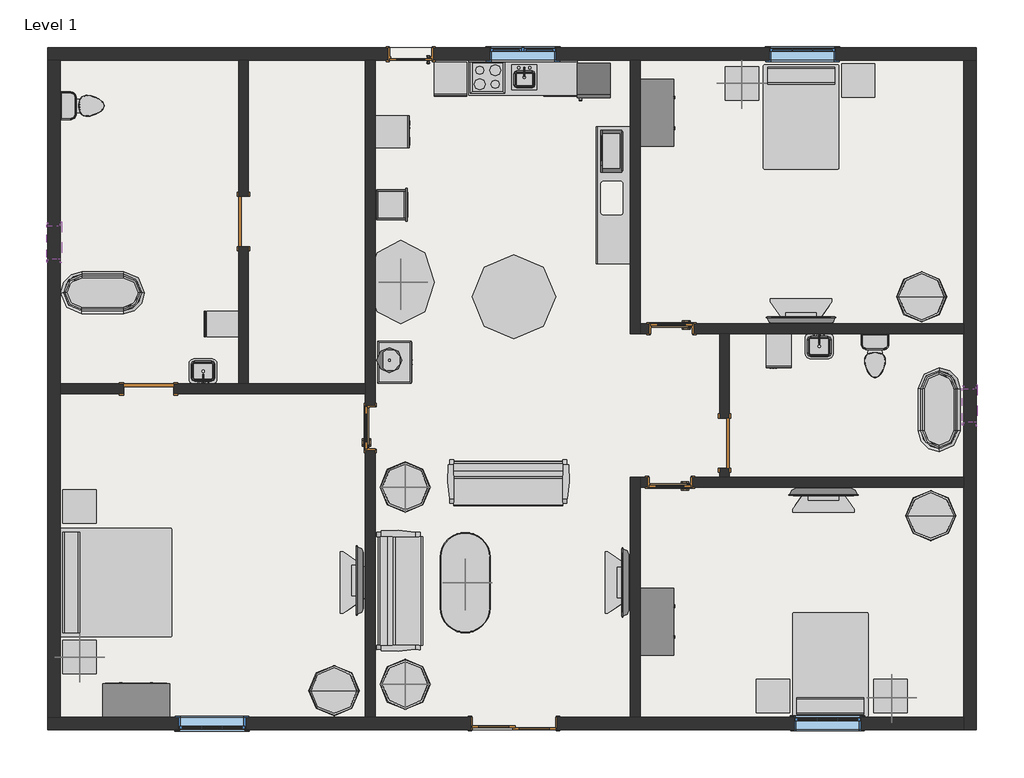
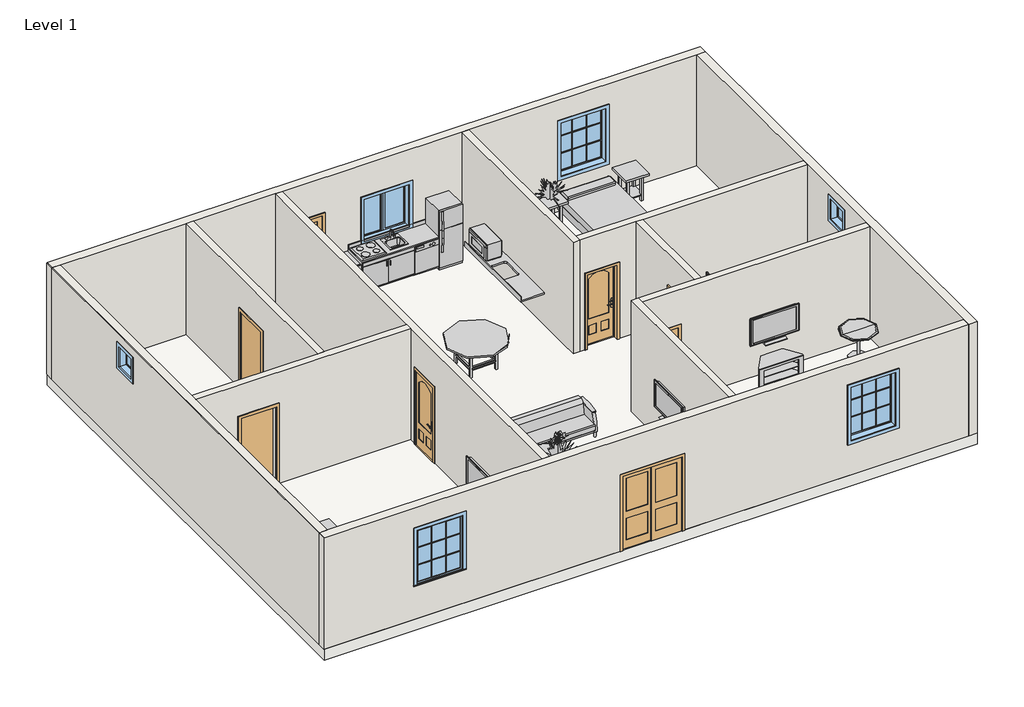
# One storey, incomplete: 33 furniture elements, 12 walls, 10 proxies, 8 doors, 8 flow terminals, 7 geographic elements, 6 windows, 1 slab.
# Revit data of these elements (continued)
# Type "Table-Dining Round w Chairs : 60\" Diameter" (continued)
#   Assembly Code = "E2020200"
#   Radius = 2' - 6"
#   Diameter = 5' - 0"
#   Height = 2' - 6"
#   Chairs = 6
#   Base Material = Pine
#   Top Material = Laminate, Linen, Matte
#   Default Elevation = 0
# Type "Table-Ellipse : 60\" x 48\""
#   Assembly Code = "E2020200"
#   Half Width = 2' - 0"
#   Half Length = 2' - 6"
#   Height = 2' - 6"
#   Length = 5' - 0"
#   Width = 4' - 0"
#   Base Material = Birch
#   Top Material = Birch
#   Default Elevation = 0
# Type "Table-Night Stand : 24\" x 24\" x 30\""
#   Assembly Code = "E2020200"
#   Depth = 2' - 0"
#   Height = 2' - 6"
#   Width = 2' - 0"
#   Base Material = Birch
#   Top Material = Laminate, Ivory, Matte
#   Default Elevation = 0
# Type "Table-Round : 36\" Diameter"
#   Assembly Code = "E2020200"
#   Base Radius = 0' - 10"
#   Height = 2' - 6"
#   Radius = 1' - 6"
#   Base Material = Steel, Chrome Plated
#   Top Material = Birch
#   Default Elevation = 0
# Type "RPC Plant - Tropical"
#   built-in parameter 1005198 = "{2, 15},{39, RPC-16-FWM5-GM7X-C67P-4000-ST1L-LVER-AU},{1, 0},{1, 0},{2, 13},{1, 8},{5, Color},{1, 0},{1, 0},{3, 0.8},{3, 0.8},{3, 0.8},{1, 8},{7, BBoxMin},{1, 0},{1, 0},{1, 0},{1, 0},{1, 0},{1, 8},{7, BBoxMax},{1, 0},{1, 0},{1, 0},{1, 0},{1, 0},{2, 11},{9, RPCTypeId},{1, 0},{1, 0},{39, RPC-16-FWM5-GM7X-C67P-4000-ST1L-LVER-AU},{1, 6},{14, RPCPlantHeight},{1, 0},{1, 0},{1, 3},{2, 11},{7, keyword},{1, 0},{1, 0},{35, :RPCs:Shrubs [General]:Geometry:RPC},{2, 11},{8, category},{1, 0},{1, 0},{16, Shrubs [General]},{2, 11},{12, LocalizedUID},{1, 0},{1, 0},{10, Crane Lily},{2, 14},{6, Height},{1, 0},{1, 0},{1, 3},{1, 2},{16, Cast Reflections},{1, 0},{1, 0},{1, 0},{1, 2},{12, Cast Shadows},{1, 0},{1, 0},{1, 1},{1, 2},{9, Lock View},{1, 0},{1, 0},{1, 0},{1, 4},{5, ViewC},{1, 0},{1, 0},{1, 0},{21, assetlibrary_base.fbx},{1, 5},"
#   built-in parameter 1005195 = "RPC-16-FWM5-GM7X-C67P-4000-ST1L-LVER-AU"
#   Assembly Code = "G2050500"
#   Height = 3' - 0"
#   Default Elevation = 0
# Type "RPC Plant - Tropical : Agave - 1.5'"
#   built-in parameter 1005198 = "{2, 15},{39, RPC-16-G1GJ-63FX-7K5P-N000-ST1L-LVER-AU},{1, 0},{1, 0},{2, 13},{1, 8},{5, Color},{1, 0},{1, 0},{3, 0.8},{3, 0.8},{3, 0.8},{1, 8},{7, BBoxMin},{1, 0},{1, 0},{1, 0},{1, 0},{1, 0},{1, 8},{7, BBoxMax},{1, 0},{1, 0},{1, 0},{1, 0},{1, 0},{2, 11},{9, RPCTypeId},{1, 0},{1, 0},{39, RPC-16-G1GJ-63FX-7K5P-N000-ST1L-LVER-AU},{1, 6},{14, RPCPlantHeight},{1, 0},{1, 0},{3, 1.5},{2, 11},{7, keyword},{1, 0},{1, 0},{35, :RPCs:Plants [General]:Geometry:RPC},{2, 11},{8, category},{1, 0},{1, 0},{16, Plants [General]},{2, 11},{12, LocalizedUID},{1, 0},{1, 0},{5, Agave},{2, 14},{6, Height},{1, 0},{1, 0},{3, 1.5},{1, 2},{16, Cast Reflections},{1, 0},{1, 0},{1, 0},{1, 2},{12, Cast Shadows},{1, 0},{1, 0},{1, 1},{1, 2},{9, Lock View},{1, 0},{1, 0},{1, 0},{1, 4},{5, ViewC},{1, 0},{1, 0},{1, 0},{21, assetlibrary_base.fbx},{1, 5},"
#   built-in parameter 1005195 = "RPC-16-G1GJ-63FX-7K5P-N000-ST1L-LVER-AU"
#   Type Comments = "Agave"
#   Assembly Code = "G2050500"
#   Height = 1' - 6"
#   Default Elevation = 0
# Type "Generic - 12\""
#   Assembly Code = "B1010"
#   Function = 0
#   Layers, outside or top first: 1' - 0" no material (function 1)
# Type "Generic - 8\""
#   Assembly Code = "B2010"
#   Layers, outside or top first: 0' - 9" "Brick, Common" (function 1)
# Type "INNER WALLS"
#   Assembly Code = "B2010"
#   Layers, outside or top first: 0' - 7" "Brick, Common" (function 1)
# Type "Casement 3x3 with Trim : 48\" x 60\""
#   Type Mark = "12"
#   Construction Type Id = "GSP4R"
#   Assembly Code = "B2020100"
#   Analytic Construction = "1/8 in Pilkington single glazing"
#   Visual Light Transmittance = 0.9
#   Solar Heat Gain Coefficient = 0.78
#   Heat Transfer Coefficient (U) = 0.6496 BTU/(h·ft²·°F)
#   Height = 5' - 0"
#   Default Sill Height = 1' - 0"
#   Trim Projection - Ext. = 0' - 0 1/2"
#   Trim Projection - Int. = 0' - 0 3/4"
#   Trim Width - Exterior = 0' - 3 1/2"
#   Trim Width - Interior = 0' - 3 1/2"
#   Width = 4' - 0"
#   Window Inset = 0' - 0 3/4"
#   Define Thermal Properties by = 1
#   Glass Pane Material = Glass
#   Sash Material = Sash
#   Trim Exterior Material = Trim
#   Trim Interior Material = Trim
#   Wall Closure = (empty or 0)
# Type "Casement Dbl with Trim : 48\" x 48\""
#   Type Mark = "13"
#   Construction Type Id = "GSP4R"
#   Assembly Code = "B2020100"
#   Analytic Construction = "1/8 in Pilkington single glazing"
#   Visual Light Transmittance = 0.9
#   Solar Heat Gain Coefficient = 0.78
#   Heat Transfer Coefficient (U) = 0.6496 BTU/(h·ft²·°F)
#   Height = 4' - 0"
#   Default Sill Height = 3' - 0"
#   Trim Projection - Ext. = 0' - 0 1/2"
#   Trim Projection - Int. = 0' - 0 3/4"
#   Trim Width - Exterior = 0' - 3 1/2"
#   Trim Width - Interior = 0' - 3 1/2"
#   Width = 4' - 0"
#   Window Inset = 0' - 0 3/4"
#   Define Thermal Properties by = 1
#   Glass Pane Material = Glass
#   Sash Material = Sash
#   Trim Exterior Material = Trim
#   Trim Interior Material = Trim
#   Wall Closure = (empty or 0)
# Type "Transom with Trim : 24\" x 24\""
#   Type Mark = "16"
#   Construction Type Id = "GSP4R"
#   Assembly Code = "B2020100"
#   Analytic Construction = "1/8 in Pilkington single glazing"
#   Visual Light Transmittance = 0.9
#   Solar Heat Gain Coefficient = 0.78
#   Heat Transfer Coefficient (U) = 0.6496 BTU/(h·ft²·°F)
#   Height = 2' - 0"
#   Default Sill Height = 7' - 1"
#   Trim Projection - Ext. = 0' - 0 1/2"
#   Trim Projection - Int. = 0' - 0 3/4"
#   Trim Width - Exterior = 0' - 3 1/2"
#   Trim Width - Interior = 0' - 3 1/2"
#   Width = 2' - 0"
#   Window Inset = 0' - 0 3/4"
#   Define Thermal Properties by = 1
#   Glass Pane Material = Glass
#   Sash Material = Sash
#   Trim Exterior Material = Trim
#   Trim Interior Material = Trim
#   Wall Closure = (empty or 0)
# Elements 1, 2 (IfcBuildingElementProxy, "18\" x 24\" x 34 1/2\"")
#   Phase Created = New Construction
#   Materials on its faces: "Steel, Paint Finish, Ivory, Matte", "Plastic, Opaque Black"
# Element 3 (IfcBuildingElementProxy, "Cook Top-4 Unit2 : 22\" x 20\"")
#   Phase Created = New Construction
#   Materials on its faces: "Steel, Chrome Plated", "Steel, Polished"
# Elements 4, 5 (IfcBuildingElementProxy, "Dishwasher : 23\" x 23 11/16\" x 33 1/2\"")
#   Phase Created = New Construction
#   Materials on its faces: "Steel, Paint Finish, Ivory, Glossy", "Plastic, Opaque Black"
# Element 6 (IfcBuildingElementProxy, "Dishwasher : 24\" x 24\" x 34\"")
#   Phase Created = New Construction
#   Materials on its faces: "Steel, Paint Finish, Ivory, Glossy", "Plastic, Opaque Black"
# Element 7 (IfcBuildingElementProxy, "Kitchenette - Medium : Kitchenette - Medium")
#   Phase Created = New Construction
#   Materials on its faces: "Cabinets", "Cabinets - Handles"
# Element 8 (IfcBuildingElementProxy, "Microwave : 30\" x 16\" x 18\"")
#   Phase Created = New Construction
#   Materials on its faces: "Laminate, Ivory, Matte", "Glass"
# Element 9 (IfcBuildingElementProxy, "Oven Double-Built-in : 21 1/2\" x 39 1/4\" x 21\"")
#   Phase Created = New Construction
#   Materials on its faces: "Steel", "Metal - Stainless Steel, Polished", "Glass"
# Element 10 (IfcBuildingElementProxy, "Refrigerator : 24\" x 25\" LH")
#   Phase Created = New Construction
#   Materials on its faces: "Steel, Paint Finish, Ivory, Glossy", "Steel, Chrome Plated"
# Elements 11, 12, 13 (IfcDoor, "30\" x 80\"")
#   Threshold Offset = 0' - 0 1/2"
#   Swing Angle = 90.00°
#   Door Offset = 0' - 0"
#   Threshold = yes
#   Exterior Trim = yes
#   Phase Created = New Construction
#   Materials on its faces: "Cherry", "Aluminum", "Glass"
# Element 14 (IfcDoor, "Door-Interior-Double-Sliding-2_Panel-Wood : 60\" x 80\"")
#   Phase Created = New Construction
#   Materials on its faces: "Cherry"
# Element 15 (IfcDoor, "Door-Interior-Single-Full Glass-Wood : 30\" x 80\"")
#   Swing Angle = 90.00°
#   Show Grill = yes
#   Phase Created = New Construction
#   Materials on its faces: "Cherry", "Aluminum", "Glass"
# Elements 16, 17, 18 (IfcDoor, "Single-Flush : 36\" x 84\"")
#   Phase Created = New Construction
#   Materials on its faces: "Door - Frame", "Door - Panel"
# Element 19 (IfcFlowTerminal, "Sink Kitchen-Island : 18\" x 18\"")
#   Mark = "10"
#   Phase Created = New Construction
#   Materials on its faces: "Steel, Polished"
# Element 20 (IfcFlowTerminal, "Sink Vanity-Round : 19\" x 19\"")
#   Mark = "11"
#   Phase Created = New Construction
#   Materials on its faces: "Porcelain, Linen", "Steel, Polished"
# Element 21 (IfcFlowTerminal, "Sink Vanity-Square : 20\" x 18\"")
#   Mark = "1"
#   Phase Created = New Construction
#   Materials on its faces: "Porcelain, Linen", "Steel, Polished"
# Element 22 (IfcFlowTerminal, "Sink Vanity-Square : 20\" x 18\"")
#   Mark = "9"
#   Phase Created = New Construction
#   Materials on its faces: "Porcelain, Linen", "Steel, Polished"
# Element 23 (IfcFlowTerminal, "Toilet-Domestic-3D : Toilet-Domestic-3D")
#   Mark = "2"
#   Phase Created = New Construction
#   Materials on its faces: "Porcelain, Linen", "Laminate, Linen, Matte"
# Element 24 (IfcFlowTerminal, "Toilet-Domestic-3D : Toilet-Domestic-3D")
#   Mark = "8"
#   Phase Created = New Construction
#   Materials on its faces: "Porcelain, Linen", "Laminate, Linen, Matte"
# Element 25 (IfcFlowTerminal, "Tub-Free Standing-3D : 30\" x 60\"")
#   Mark = "6"
#   Phase Created = New Construction
#   Materials on its faces: "Porcelain, Ivory"
# Element 26 (IfcFlowTerminal, "Tub-Free Standing-3D : 30\" x 60\"")
#   Mark = "7"
#   Phase Created = New Construction
#   Materials on its faces: "Porcelain, Ivory"
# Element 27 (IfcFurniture, "Base Cabinet-Double Door Sink Unit : 30\"")
#   Phase Created = New Construction
#   Materials on its faces: "Cabinets", "Cabinets - Handles"
# Elements 28, 29 (IfcFurniture, "Bed-Standard.0001 : Double 54\" x 75\"")
#   Phase Created = New Construction
#   Materials on its faces: "Linen, White", "Steel, Chrome Plated"
# Element 30 (IfcFurniture, "Bed-Standard.0001 : King 78\" x 80\"")
#   Phase Created = New Construction
#   Materials on its faces: "Linen, White", "Steel, Chrome Plated"
# Element 31 (IfcFurniture, "Counter Top w Sink Hole : 0600mm Depth")
#   Sink Opening Width = 1' - 11 1/8"
#   Sink Opening Depth = 1' - 2 7/8"
#   Sink Location To Wall = 0' - 3 15/16"
#   Sink Location = 3' - 11 1/4"
#   Length = 8' - 2 7/16"
#   Phase Created = New Construction
#   Materials on its faces: "Counter Top"
# Element 32 (IfcFurniture, "Counter Top w Sink Hole : 24\" Depth")
#   Sink Opening Depth = 1' - 2"
#   Sink Location To Wall = 0' - 6"
#   Length = 6' - 6"
#   Sink Location = 3' - 4"
#   Sink Opening Width = 1' - 4"
#   Phase Created = New Construction
#   Materials on its faces: "Counter Top"
# Elements 33, 34, 35 (IfcFurniture, "Dresser : 48\" x 72\" x 24\"")
#   Phase Created = New Construction
#   Materials on its faces: "Laminate, Ivory, Matte", "Cherry", "Laminate - Ivory, Glossy"
# Elements 36, 37 (IfcFurniture, "Sofa-Pensi : 84\"")
#   Phase Created = New Construction
#   Materials on its faces: "Cherry", "Linen, Beige", "Steel, Chrome Plated"
# Elements 38, 39, 40, 41 (IfcFurniture, "TV - Flat Screen : 50\"")
#   Stand = yes
#   Phase Created = New Construction
#   Materials on its faces: "TV - Black", "TV - Glass", "TV - Screen"
# Elements 42, 43, 44, 45 (IfcFurniture, "TV Stand : TV Stand")
#   Phase Created = New Construction
#   Materials on its faces: "Melamine - Gray", "Glass - Shelves"
# Element 46 (IfcFurniture, "Table-Dining Oval : 36\" x 72\"")
#   Phase Created = New Construction
#   Materials on its faces: "Steel, Chrome Plated", "Glass - Clear, Grey"
# Element 47 (IfcFurniture, "Table-Dining Round w Chairs : 60\" Diameter")
#   Phase Created = New Construction
#   Materials on its faces: "Pine", "Laminate, Linen, Matte"
# Element 48 (IfcFurniture, "Table-Ellipse : 60\" x 48\"")
#   Phase Created = New Construction
#   Materials on its faces: "Birch"
# Elements 49, 50, 51, 52, 53, 54 (IfcFurniture, "Table-Night Stand : 24\" x 24\" x 30\"")
#   Phase Created = New Construction
#   Materials on its faces: "Birch", "Laminate, Ivory, Matte"
# Elements 55, 56, 57, 58, 59 (IfcFurniture, "Table-Round : 36\" Diameter")
#   Phase Created = New Construction
#   Materials on its faces: "Steel, Chrome Plated", "Birch"
# Elements 60, 61 (IfcGeographicElement, "RPC Plant - Tropical")
#   Phase Created = New Construction
# Elements 62, 63, 64, 65, 66 (IfcGeographicElement, "RPC Plant - Tropical : Agave - 1.5'")
#   Phase Created = New Construction
# Element 67 (IfcSlab, "Generic - 12\"")
#   Height Offset From Level = 0' - 0"
#   Phase Created = New Construction
#   Materials on its faces: "Default Floor"
# Elements 68, 69, 70, 71 (IfcWall, "Generic - 8\"")
#   Top Offset = 0' - 0"
#   Base Offset = 0' - 0"
#   Unconnected Height = 10' - 0"
#   wall height = 10' - 0"
#   Phase Created = New Construction
#   Base Constraint = Level 1
#   Materials on its faces: "Brick, Common"
# Elements 72, 73, 74, 75, 76, 77, 78, 79 (IfcWall, "INNER WALLS")
#   Top Offset = 0' - 0"
#   Base Offset = 0' - 0"
#   Unconnected Height = 10' - 0"
#   wall height = 10' - 0"
#   Phase Created = New Construction
#   Base Constraint = Level 1
#   Materials on its faces: "Brick, Common"
# Element 80 (IfcWindow, "Casement 3x3 with Trim : 48\" x 60\"")
#   Mark = "1"
#   Phase Created = New Construction
#   Materials on its faces: "Sash", "Glass", "Trim"
# Element 81 (IfcWindow, "Casement 3x3 with Trim : 48\" x 60\"")
#   Mark = "3"
#   Phase Created = New Construction
#   Materials on its faces: "Sash", "Glass", "Trim"
# Element 82 (IfcWindow, "Casement 3x3 with Trim : 48\" x 60\"")
#   Mark = "2"
#   Phase Created = New Construction
#   Materials on its faces: "Sash", "Glass", "Trim"
# Element 83 (IfcWindow, "Casement Dbl with Trim : 48\" x 48\"")
#   Mark = "4"
#   Phase Created = New Construction
#   Materials on its faces: "Sash", "Trim", "Glass"
# Element 84 (IfcWindow, "Transom with Trim : 24\" x 24\"")
#   Mark = "5"
#   Phase Created = New Construction
#   Materials on its faces: "Sash", "Trim", "Glass"
# Element 85 (IfcWindow, "Transom with Trim : 24\" x 24\"")
#   Mark = "6"
#   Phase Created = New Construction
#   Materials on its faces: "Sash", "Trim", "Glass"
# Materials
#   "Plastic, Opaque Black": class "Plastic", colour RGB 0 0 0, transparency 0.7, Description = "Plastic, generic, opaque black", Cost = 0
#   "Steel, Paint Finish, Ivory, Matte": class "Metal", colour RGB 247 247 239, transparency 0, Description = "Steel, paint finish, ivory, matte", Cost = 0
#   "Steel, Chrome Plated": class "Metal", colour RGB 17 17 17, transparency 0, Description = "Chromiuim plated steel", Cost = 0
#   "Steel, Polished": class "Metal", colour RGB 57 57 57, transparency 0, Description = "Polished steel", Cost = 0
#   "Steel, Paint Finish, Ivory, Glossy": class "Metal", colour RGB 247 247 239, transparency 0, Description = "Steel, paint finish, ivory, glossy", Cost = 0
#   "Cabinets": colour RGB 249 249 249, transparency 0
#   "Cabinets - Handles": class "Metal", colour RGB 57 57 57, transparency 0
#   "Laminate, Ivory, Matte": class "Plastic", colour RGB 247 247 239, transparency 0, Description = "Plastic Laminate - Ivory, Matte", Cost = 0
#   "Metal - Stainless Steel, Polished": class "Metal", colour RGB 216 216 216, transparency 0
#   "Cherry": class "Wood", colour RGB 226 177 128, transparency 0, Description = "Prunus Serotina", Cost = 0
#   "Glass": class "Glass", colour RGB 0 128 192, transparency 0.75, Description = "Soda Lime Glass", Cost = 0
#   "Aluminum": class "Metal", colour RGB 247 247 247, transparency 0, Description = "Aluminum 6061", Cost = 0
#   "Door - Panel": class "Wood", colour RGB 210 159 95, transparency 0
#   "Door - Frame": colour RGB 118 70 51, transparency 0
#   "Porcelain, Linen": class "Ceramic", colour RGB 249 239 230, transparency 0, Description = "Porcelain, linen", Cost = 0
#   "Laminate, Linen, Matte": class "Plastic", colour RGB 249 239 230, transparency 0, Description = "Plastic Laminate - Linen, Matte", Cost = 0
#   "Porcelain, Ivory": class "Ceramic", colour RGB 247 247 239, transparency 0, Description = "Porcelain, ivory", Cost = 0
#   "Linen, White": class "Textile", colour RGB 247 247 239, transparency 0, Description = "Linen, white", Cost = 0
#   "Laminate - Ivory, Glossy": colour RGB 247 247 239, transparency 0
#   "Linen, Beige": class "Textile", colour RGB 249 239 230, transparency 0, Description = "Linen, beige", Cost = 0
#   "Melamine - Gray": class "Wood", colour RGB 49 49 49, transparency 0
#   "Glass - Clear, Grey": class "Glass", colour RGB 252 255 255, transparency 0.64
#   "Pine": class "Wood", colour RGB 223 192 134, transparency 0, Description = "Pinus Echinata", Cost = 0
#   "Birch": class "Wood", colour RGB 224 178 126, transparency 0, Description = "Betula Alleghaniensis", Cost = 0
#   "Brick, Common": class "Masonry", colour RGB 170 98 104, transparency 0, Description = "Common brick", Cost = 0
#   "Sash": class "Wood", colour RGB 224 178 126, transparency 0
#   "Trim": class "Wood", colour RGB 224 178 126, transparency 0
#   "Steel": class "Metal", colour RGB 247 247 247, transparency 0, Description = "Steel, mill finish", Cost = 0
#   "Counter Top": class "Wood", colour RGB 226 177 128, transparency 0
#   "TV - Black": colour RGB 49 49 49, transparency 0
#   "TV - Glass": colour RGB 157 157 157, transparency 0.9
#   "TV - Screen": colour RGB 0 0 0, transparency 0
#   "Glass - Shelves": class "Glass", colour RGB 167 167 167, transparency 0.9
#   "Default Floor": colour RGB 128 128 128, transparency 0
# Room at (3451.585, 2682.46) mm, phase "New Construction", upper level "Level 1", upper offset 10' - 0", lower offset 0' - 0"
#   Number = "7"
#   Name = "BEDROOM 3"
# Room at (-8844.864, 10050.872) mm, phase "New Construction", upper level "Level 1", upper offset 10' - 0", lower offset 0' - 0"
#   Number = "1"
#   Name = "ENSUITE BATH"
# Room at (-7963.549, 3944.615) mm, phase "New Construction", upper level "Level 1", upper offset 10' - 0", lower offset 0' - 0"
#   Number = "2"
#   Name = "MASTER BEDROOM"
# Room at (-2570.737, 3147.235) mm, phase "New Construction", upper level "Level 1", upper offset 10' - 0", lower offset 0' - 0"
#   Number = "3"
#   Name = "LIVING ROOM"
# Room at (-2570.737, 10050.872) mm, phase "New Construction", upper level "Level 1", upper offset 10' - 0", lower offset 0' - 0"
#   Number = "4"
#   Name = "OPEN KITCHEN"
# Room at (2926.992, 10680.383) mm, phase "New Construction", upper level "Level 1", upper offset 10' - 0", lower offset 0' - 0"
#   Number = "5"
#   Name = "BEDROOM 2"
# Room at (3808.308, 6210.855) mm, phase "New Construction", upper level "Level 1", upper offset 10' - 0", lower offset 0' - 0"
#   Number = "6"
#   Name = "SHARED BATH"
